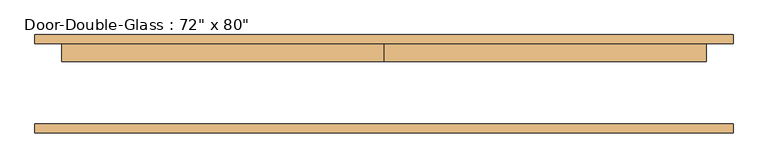
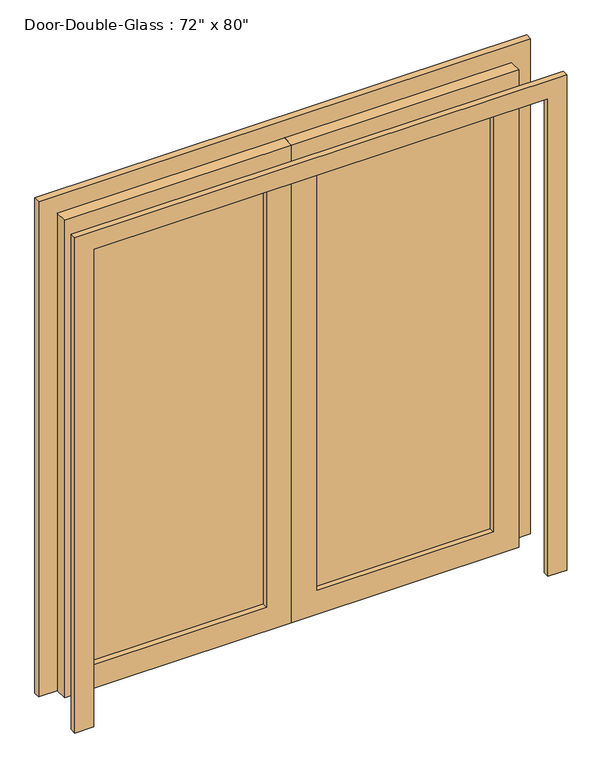
"""IFC4 building model written with IfcOpenShell, lengths in millimetres: door geometry."""

from ifc_helpers import new_model, si_unit, frame, origin, place, context, project, spatial, polyline, outline, extrude, source, transform, mapped, element, save


def door_4594e60e(model_context):
    return source(origin(), model_context, "Body", "SweptSolid", [
        extrude(outline(polyline([(2032.0, 914.4), (2032.0, 0.0), (0.0, 0.0), (0.0, 914.4), (2032.0, 914.4)]), holes=[polyline([(1930.4, 812.8), (101.6, 812.8), (101.6, 101.6), (1930.4, 101.6), (1930.4, 812.8)])]), frame((0.0, 65.88125, 0.0), z_axis=(0.0, 1.0, 0.0), x_axis=(0.0, 0.0, 1.0)), (0.0, 0.0, 1.0), 50.8),
        extrude(outline(polyline([(2032.0, -914.4), (0.0, -914.4), (0.0, 0.0), (2032.0, 0.0), (2032.0, -914.4)]), holes=[polyline([(1930.4, -812.8), (1930.4, -101.6), (101.6, -101.6), (101.6, -812.8), (1930.4, -812.8)])]), frame((0.0, 65.88125, 0.0), z_axis=(0.0, 1.0, 0.0), x_axis=(0.0, 0.0, 1.0)), (0.0, 0.0, 1.0), 50.8),
        extrude(outline(polyline([(-812.8, 94.45625), (-101.6, 94.45625), (-101.6, 88.10625), (-812.8, 88.10625), (-812.8, 94.45625)])), frame((0.0, 0.0, 101.6), z_axis=(0.0, 0.0, 1.0), x_axis=(1.0, 0.0, 0.0)), (0.0, 0.0, 1.0), 1828.8),
        extrude(outline(polyline([(101.6, 94.45625), (812.8, 94.45625), (812.8, 88.10625), (101.6, 88.10625), (101.6, 94.45625)])), frame((0.0, 0.0, 101.6), z_axis=(0.0, 0.0, 1.0), x_axis=(1.0, 0.0, 0.0)), (0.0, 0.0, 1.0), 1828.8),
        extrude(outline(polyline([(0.0, 990.6), (2108.2, 990.6), (2108.2, -990.6), (0.0, -990.6), (0.0, -914.4), (2032.0, -914.4), (2032.0, 914.4), (0.0, 914.4), (0.0, 990.6)])), frame((0.0, -137.31875, 0.0), z_axis=(0.0, 1.0, 0.0), x_axis=(0.0, 0.0, 1.0)), (0.0, 0.0, 1.0), 25.4),
        extrude(outline(polyline([(0.0, 990.6), (2108.2, 990.6), (2108.2, -990.6), (0.0, -990.6), (0.0, -914.4), (2032.0, -914.4), (2032.0, 914.4), (0.0, 914.4), (0.0, 990.6)])), frame((0.0, 116.68125, 0.0), z_axis=(0.0, 1.0, 0.0), x_axis=(0.0, 0.0, 1.0)), (0.0, 0.0, 1.0), 25.4),
    ])


if __name__ == "__main__":
    model = new_model("IFC4")
    model_context = context("Model", 3, world=origin())
    ifc_project = project(units=[si_unit("LENGTHUNIT", "METRE", prefix="MILLI")], contexts=[model_context])
    site = spatial("IfcSite", under=ifc_project)
    building = spatial("IfcBuilding", under=site)
    placement = place(None, origin())
    door_shape = door_4594e60e(model_context)
    element("IfcDoor", 1, ObjectType="Door-Double-Glass : 72\" x 80\"", at=placement, inside=building, context=model_context, shape_type="MappedRepresentation", body=[
        mapped(door_shape, transform((0.0, 0.0, 0.0), x_axis=(1.0, 0.0, 0.0), y_axis=(0.0, 1.0, 0.0), z_axis=(0.0, 0.0, 1.0))),
    ])
    save(model, "model.ifc")

# Revit data of these elements
# Type "Door-Double-Glass : 72\" x 80\""
#   Type Mark = "12"
#   Construction Type Id = "opn-d45"
#   Assembly Code = "C1020"
#   Analytic Construction = "Wood frame, double glass door "
#   W = 3' - 0"
#   Thickness = 0' - 2"
#   Thermal Resistance (R) = 1.8150 (h·ft²·°F)/BTU
#   Swing Angle [instance default] = 90.00°
#   Heat Transfer Coefficient (U) = 0.5510 BTU/(h·ft²·°F)
#   Height = 6' - 8"
#   Bottom Rail = 0' - 4"
#   Top Rail = 0' - 4"
#   Stiles = 0' - 4"
#   Trim Projection = 0' - 1"
#   Trim Width = 0' - 3"
#   Width = 6' - 0"
#   Define Thermal Properties by = 1
#   Glazing = Glass
#   Panel Material = Wood - Birch - Solid Stained Light Low Gloss
#   Trim Material = Paint - Sienna
#   Visual Light Transmittance = 0
#   Solar Heat Gain Coefficient = 0
#   Function = (empty or 0)
#   Wall Closure = (empty or 0)
# Element 1 (IfcDoor, "Door-Double-Glass : 72\" x 80\"")
#   Materials on its faces: "Wood - Birch - Solid Stained Light Low Gloss", "Paint - Sienna", "Glass"
# Materials
#   "Glass": class "Glass", colour RGB 0 128 192, transparency 0.75, Description = "Soda Lime Glass", Cost = 0
#   "Wood - Birch - Solid Stained Light Low Gloss": class "Wood", colour RGB 210 159 95, transparency 0, Cost = 0
#   "Paint - Sienna": colour RGB 118 70 51, transparency 0, Cost = 0
